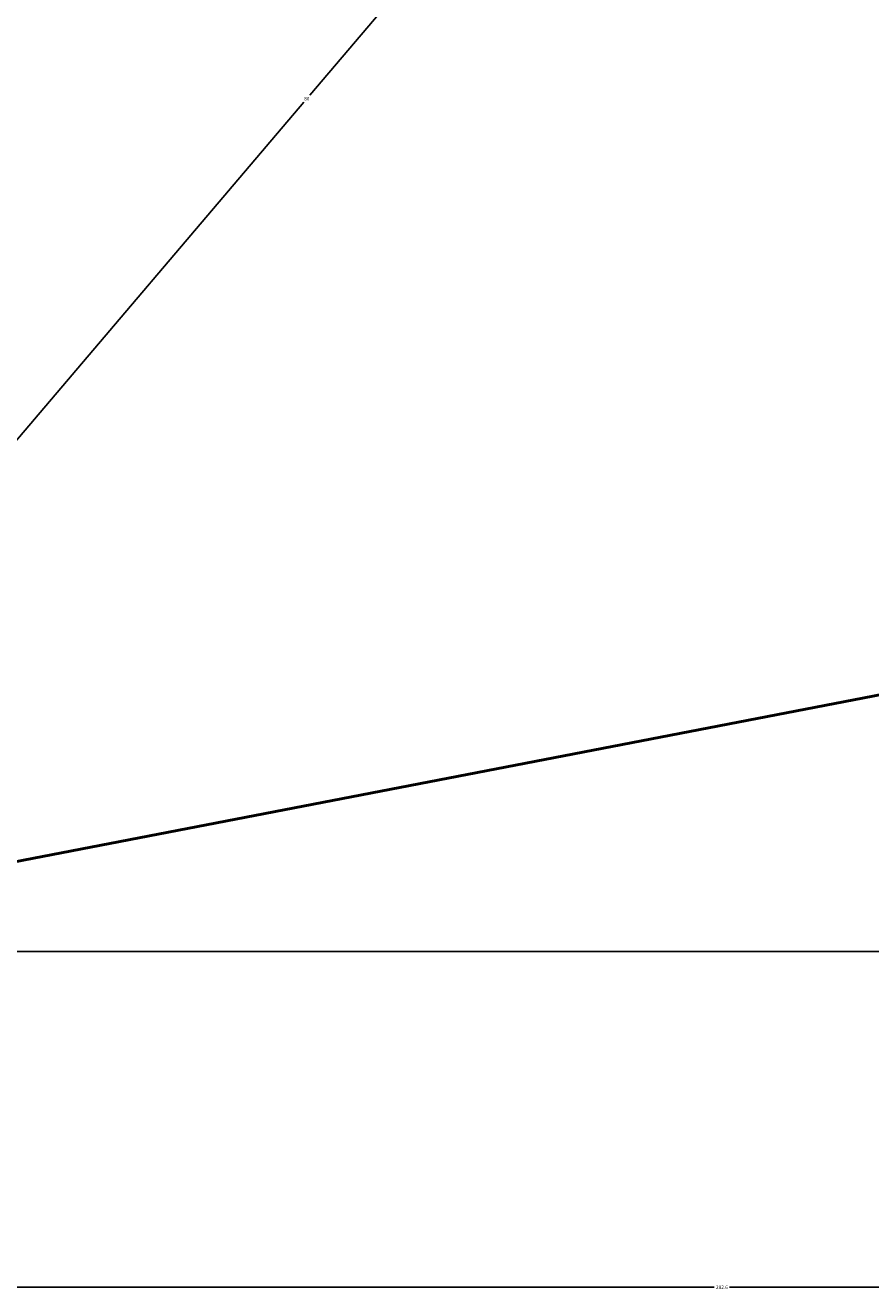
# Model space of a CAD drawing. Units: inches. Extents: x 457 to 775, y 319 to 541.
# Tile 5 of 12: x 580 to 623, y 319 to 385. Entities that reach past the tile are written whole.
import ezdxf

# ---------------------------------------------------------------- set-up
doc = ezdxf.new("R2010")
doc.units = ezdxf.units.IN
doc.header["$MEASUREMENT"] = 0
doc.layers.add('M-DIMS', color=2, linetype='Continuous', lineweight=18)
doc.layers.add('M-OUTL', color=7, linetype='Continuous', lineweight=50)
doc.styles.get("Standard").update_dxf_attribs({"font": 'arial.ttf'})
doc.dimstyles.get("Standard").update_dxf_attribs({"dimtxt": 0.18, "dimasz": 0.18, "dimexe": 0.18, "dimexo": 0.0625, "dimgap": 0.09, "dimtad": 0, "dimtih": 1, "dimtoh": 1, "dimdec": 4, "dimzin": 0, "dimdsep": 46, "dimtxsty": 'Standard', "dimcen": 0.09, "dimadec": 0, "dimazin": 0, "dimtfac": 1, "dimtdec": 4, "dimtofl": 0, "dimtmove": 0, "dimatfit": 3, "dimfxl": 1, "dimtolj": 1, "dimtzin": 0, "dimarcsym": 0})

# ---------------------------------------------------------------- blocks, each defined once
blk = doc.blocks.new('*D2')
at = {"layer": 'Defpoints', "color": 0, "transparency": 16777216}
for p in [(756.931, 375.696), (474.306, 336.696), (756.931, 319.296)]:
    blk.add_point(p, dxfattribs=at)
at = {"layer": 'M-DIMS', "color": 0, "lineweight": -2, "transparency": 16777216}
for p, q in [((756.931, 375.634), (756.931, 319.116)), ((474.306, 336.634), (474.306, 319.116)), ((474.486, 319.296), (615.223, 319.296)), ((756.751, 319.296), (616.014, 319.296))]:
    blk.add_line(p, q, dxfattribs=at)
at = {"layer": 'M-DIMS', "color": 0, "transparency": 16777216}
for points in [[(474.486, 319.326), (474.486, 319.266), (474.306, 319.296)], [(756.751, 319.326), (756.751, 319.266), (756.931, 319.296)]]:
    blk.add_solid(points, dxfattribs=at)
at = {"layer": 'M-DIMS', "color": 0, "transparency": 16777216, "insert": (615.619, 319.296), "char_height": 0.18, "attachment_point": 5}
blk.add_mtext('\\A1;282.6', dxfattribs=at)
blk = doc.blocks.new('*D3')
at = {"layer": 'Defpoints', "color": 0, "transparency": 16777216}
for p in [(456.906, 523.213), (646.001, 523.213), (474.306, 336.696)]:
    blk.add_point(p, dxfattribs=at)
at = {"layer": 'M-DIMS', "color": 0, "lineweight": -2, "transparency": 16777216}
for p, q in [((645.939, 523.213), (456.726, 523.213)), ((456.906, 523.033), (456.906, 430.136)), ((456.906, 336.876), (456.906, 429.773)), ((474.244, 336.696), (456.726, 336.696))]:
    blk.add_line(p, q, dxfattribs=at)
at = {"layer": 'M-DIMS', "color": 0, "transparency": 16777216}
for points in [[(456.876, 523.033), (456.936, 523.033), (456.906, 523.213)], [(456.876, 336.876), (456.936, 336.876), (456.906, 336.696)]]:
    blk.add_solid(points, dxfattribs=at)
at = {"layer": 'M-DIMS', "color": 0, "transparency": 16777216, "insert": (456.906, 429.954), "char_height": 0.18, "attachment_point": 5}
blk.add_mtext('\\A1;186.5', dxfattribs=at)
blk = doc.blocks.new('*D9')
at = {"layer": 'Defpoints', "color": 0, "transparency": 16777216}
for p in [(756.931, 375.696), (774.331, 375.696), (554.931, 336.696)]:
    blk.add_point(p, dxfattribs=at)
at = {"layer": 'M-DIMS', "color": 0, "lineweight": -2, "transparency": 16777216}
for p, q in [((756.994, 375.696), (774.511, 375.696)), ((774.331, 375.516), (774.331, 356.378)), ((774.331, 336.876), (774.331, 356.014)), ((554.994, 336.696), (774.511, 336.696))]:
    blk.add_line(p, q, dxfattribs=at)
at = {"layer": 'M-DIMS', "color": 0, "transparency": 16777216}
for points in [[(774.301, 375.516), (774.361, 375.516), (774.331, 375.696)], [(774.301, 336.876), (774.361, 336.876), (774.331, 336.696)]]:
    blk.add_solid(points, dxfattribs=at)
at = {"layer": 'M-DIMS', "color": 0, "transparency": 16777216, "insert": (774.331, 356.196), "char_height": 0.18, "attachment_point": 5}
blk.add_mtext('\\A1;39', dxfattribs=at)
blk = doc.blocks.new('*D17')
at = {"layer": 'Defpoints', "color": 0, "transparency": 16777216}
for p in [(606.761, 540.613), (606.761, 422.636), (554.931, 361.696)]:
    blk.add_point(p, dxfattribs=at)
at = {"layer": 'M-DIMS', "color": 0, "lineweight": -2, "transparency": 16777216}
for p, q in [((554.931, 361.759), (554.931, 540.793)), ((555.111, 540.613), (580.452, 540.613)), ((606.581, 540.613), (581.24, 540.613)), ((606.761, 422.698), (606.761, 540.793))]:
    blk.add_line(p, q, dxfattribs=at)
at = {"layer": 'M-DIMS', "color": 0, "transparency": 16777216}
for points in [[(555.111, 540.643), (555.111, 540.583), (554.931, 540.613)], [(606.581, 540.643), (606.581, 540.583), (606.761, 540.613)]]:
    blk.add_solid(points, dxfattribs=at)
at = {"layer": 'M-DIMS', "color": 0, "transparency": 16777216, "insert": (580.846, 540.613), "char_height": 0.18, "attachment_point": 5}
blk.add_mtext('\\A1;51.83', dxfattribs=at)
blk = doc.blocks.new('*D18')
at = {"layer": 'Defpoints', "color": 0, "transparency": 16777216}
for p in [(606.761, 422.636), (554.931, 361.696), (568.185, 350.423)]:
    blk.add_point(p, dxfattribs=at)
at = {"layer": 'M-DIMS', "color": 0, "lineweight": -2, "transparency": 16777216}
for p, q in [((606.809, 422.595), (620.153, 411.246)), ((619.899, 411.226), (594.255, 381.075)), ((568.302, 350.56), (593.946, 380.711)), ((554.979, 361.656), (568.323, 350.306))]:
    blk.add_line(p, q, dxfattribs=at)
at = {"layer": 'M-DIMS', "color": 0, "transparency": 16777216}
for points in [[(619.876, 411.245), (619.922, 411.206), (620.015, 411.363)], [(568.279, 350.58), (568.325, 350.541), (568.185, 350.423)]]:
    blk.add_solid(points, dxfattribs=at)
at = {"layer": 'M-DIMS', "color": 0, "transparency": 16777216, "insert": (594.1, 380.893), "char_height": 0.18, "attachment_point": 5}
blk.add_mtext('\\A1;80', dxfattribs=at)

msp = doc.modelspace()

# ---------------------------------------------------------------- linework, layer by layer
at = {"layer": 'M-OUTL'}
msp.add_line((554.931, 336.696), (756.931, 375.696), dxfattribs=at)

# ---------------------------------------------------------------- dimensions: what is measured, and where the dimension line sits
at = {"layer": 'M-DIMS'}
for base, p1, p2, override, picture, middle in [((606.761, 540.613), (554.931, 361.696), (606.761, 422.636), {"dimdec": 2, "dimlfac": 1, "dimrnd": 0, "dimzin": 0, "dimdsep": 46, "dimlunit": 2}, '*D17', (580.846, 540.613)), ((756.931, 319.296), (474.306, 336.696), (756.931, 375.696), {"dimdec": 1, "dimlfac": 1, "dimrnd": 0, "dimzin": 0, "dimdsep": 46, "dimlunit": 2}, '*D2', (615.619, 319.296))]:
    dim = msp.add_linear_dim(base=base, p1=p1, p2=p2, dimstyle='Standard', override=override, dxfattribs=at)
    dim.commit()
    dim.dimension.update_dxf_attribs({"geometry": picture, "text_midpoint": middle})
for base, p1, p2, angle, override, picture, middle in [((456.906, 523.213), (474.306, 336.696), (646.001, 523.213), 90, {"dimdec": 1, "dimlfac": 1, "dimrnd": 0, "dimzin": 0, "dimdsep": 46, "dimlunit": 2}, '*D3', (456.906, 429.954)), ((568.185, 350.423), (606.761, 422.636), (554.931, 361.696), 229.61848, {"dimdec": 0, "dimlfac": 1, "dimrnd": 0, "dimzin": 0, "dimdsep": 46, "dimlunit": 2}, '*D18', (594.1, 380.893)), ((774.331, 375.696), (554.931, 336.696), (756.931, 375.696), 90, {"dimdec": 0, "dimlfac": 1, "dimrnd": 0, "dimzin": 0, "dimdsep": 46, "dimlunit": 2}, '*D9', (774.331, 356.196))]:
    dim = msp.add_linear_dim(base=base, p1=p1, p2=p2, angle=angle, dimstyle='Standard', override=override, dxfattribs=at)
    dim.commit()
    dim.dimension.update_dxf_attribs({"geometry": picture, "text_midpoint": middle})

doc.saveas('drawing.dxf')
